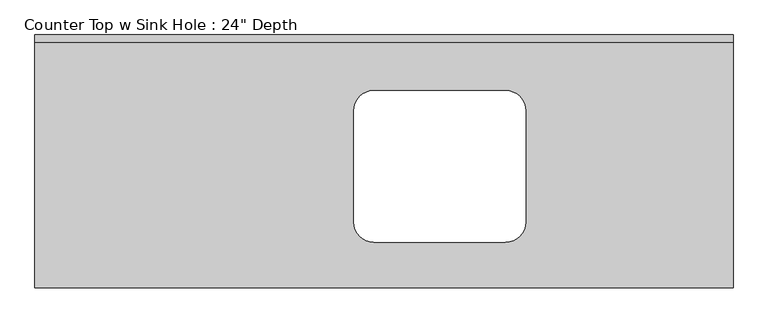
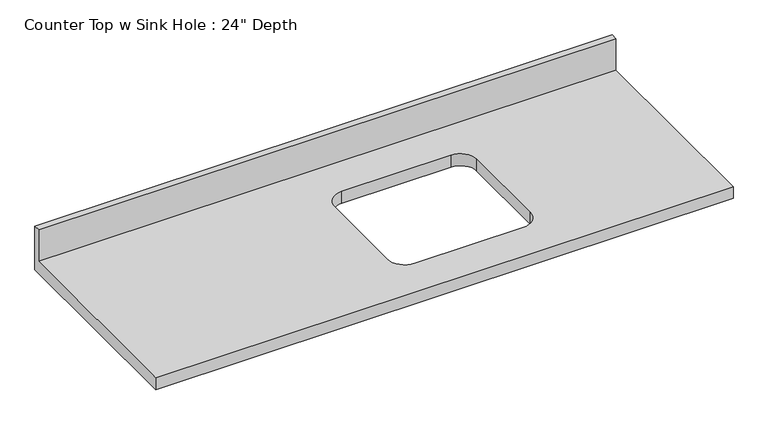
"""IFC4 building model written with IfcOpenShell, lengths in millimetres: furniture geometry."""

from ifc_helpers import new_model, si_unit, frame, origin, place, context, project, spatial, polyline, circle_curve, source, transform, mapped, element, save
from ifc_brep_helpers import plane_surface, revolved_surface, advanced_brep


def furniture_f14924cf(model_context):
    return source(origin(), model_context, "Body", "AdvancedBrep", [
        advanced_brep(
        [(-1200.4622951, -635.0, 914.4), (552.1377049, -635.0, 914.4), (552.1377049, -19.05, 914.4), (-1200.4622951, -19.05, 914.4), (-349.5622951, -139.7, 914.4), (-19.3622951, -139.7, 914.4), (31.4377049, -190.5, 914.4), (31.4377049, -469.9, 914.4), (-19.3622951, -520.7, 914.4), (-349.5622951, -520.7, 914.4), (-400.3622951, -469.9, 914.4), (-400.3622951, -190.5, 914.4), (552.1377049, 0.0, 876.3), (552.1377049, -635.0, 876.3), (-1200.4622951, -635.0, 876.3), (-1200.4622951, 0.0, 876.3), (-19.3622951, -139.7, 876.3), (-349.5622951, -139.7, 876.3), (-400.3622951, -190.5, 876.3), (-400.3622951, -469.9, 876.3), (-349.5622951, -520.7, 876.3), (-19.3622951, -520.7, 876.3), (31.4377049, -469.9, 876.3), (31.4377049, -190.5, 876.3), (-1200.4622951, 0.0, 1016.0), (552.1377049, 0.0, 1016.0), (-1200.4622951, -19.05, 1016.0), (552.1377049, -19.05, 1016.0)],
        [
            (0, 1),
            (1, 2),
            (2, 3),
            (3, 0),
            (4, 5),
            (5, 6, circle_curve(frame((-19.3622951, -190.5, 914.4), z_axis=(0.0, 0.0, -1.0), x_axis=(1.0, 0.0, 0.0)), 50.8)),
            (6, 7),
            (7, 8, circle_curve(frame((-19.3622951, -469.9, 914.4), z_axis=(0.0, 0.0, -1.0), x_axis=(1.0, 0.0, 0.0)), 50.8)),
            (8, 9),
            (9, 10, circle_curve(frame((-349.5622951, -469.9, 914.4), z_axis=(0.0, 0.0, -1.0), x_axis=(1.0, 0.0, 0.0)), 50.8)),
            (10, 11),
            (11, 4, circle_curve(frame((-349.5622951, -190.5, 914.4), z_axis=(0.0, 0.0, -1.0), x_axis=(1.0, 0.0, 0.0)), 50.8)),
            (12, 13),
            (13, 14),
            (14, 15),
            (15, 12),
            (16, 17),
            (17, 18, circle_curve(frame((-349.5622951, -190.5, 876.3), z_axis=(0.0, 0.0, 1.0), x_axis=(1.0, 0.0, 0.0)), 50.8)),
            (18, 19),
            (19, 20, circle_curve(frame((-349.5622951, -469.9, 876.3), z_axis=(0.0, 0.0, 1.0), x_axis=(1.0, 0.0, 0.0)), 50.8)),
            (20, 21),
            (21, 22, circle_curve(frame((-19.3622951, -469.9, 876.3), z_axis=(0.0, 0.0, 1.0), x_axis=(1.0, 0.0, 0.0)), 50.8)),
            (22, 23),
            (23, 16, circle_curve(frame((-19.3622951, -190.5, 876.3), z_axis=(0.0, 0.0, 1.0), x_axis=(1.0, 0.0, 0.0)), 50.8)),
            (15, 24),
            (24, 25),
            (25, 12),
            (14, 0),
            (3, 26),
            (26, 24),
            (13, 1),
            (25, 27),
            (27, 2),
            (4, 17),
            (16, 5),
            (11, 18),
            (10, 19),
            (9, 20),
            (8, 21),
            (7, 22),
            (6, 23),
            (26, 27),
        ],
        [
            plane_surface(frame((-1200.4622951, 0.0, 914.4), z_axis=(0.0, 0.0, 1.0), x_axis=(-1.0, 0.0, 0.0))),
            plane_surface(frame((-1200.4622951, 0.0, 876.3), z_axis=(0.0, 0.0, -1.0), x_axis=(1.0, 0.0, 0.0))),
            plane_surface(frame((552.1377049, 0.0, 914.4), z_axis=(0.0, 1.0, 0.0), x_axis=(0.0, 0.0, -1.0))),
            plane_surface(frame((-1200.4622951, 0.0, 914.4), z_axis=(-1.0, 0.0, 0.0), x_axis=(0.0, 0.0, -1.0))),
            plane_surface(frame((-1200.4622951, -635.0, 914.4), z_axis=(0.0, -1.0, 0.0), x_axis=(0.0, 0.0, -1.0))),
            plane_surface(frame((552.1377049, -635.0, 914.4), z_axis=(1.0, 0.0, 0.0), x_axis=(0.0, 0.0, -1.0))),
            plane_surface(frame((-19.3622951, -139.7, 914.4), z_axis=(0.0, -1.0, 0.0), x_axis=(0.0, 0.0, -1.0))),
            revolved_surface(polyline([(-298.76229509999996, -190.5, 914.4), (-298.76229509999996, -190.5, 876.3)]), (-349.5622951, -190.5, 876.3), (0.0, 0.0, 1.0)),
            plane_surface(frame((-400.3622951, -190.5, 914.4), z_axis=(1.0, 0.0, 0.0), x_axis=(0.0, 0.0, -1.0))),
            revolved_surface(polyline([(-298.76229509999996, -469.9, 914.4), (-298.76229509999996, -469.9, 876.3)]), (-349.5622951, -469.9, 876.3), (0.0, 0.0, 1.0)),
            plane_surface(frame((-349.5622951, -520.7, 914.4), z_axis=(0.0, 1.0, 0.0), x_axis=(0.0, 0.0, -1.0))),
            revolved_surface(polyline([(31.437704899999996, -469.9, 914.4), (31.437704899999996, -469.9, 876.3)]), (-19.3622951, -469.9, 876.3), (0.0, 0.0, 1.0)),
            plane_surface(frame((31.4377049, -469.9, 914.4), z_axis=(-1.0, 0.0, 0.0), x_axis=(0.0, 0.0, -1.0))),
            revolved_surface(polyline([(31.437704899999996, -190.5, 914.4), (31.437704899999996, -190.5, 876.3)]), (-19.3622951, -190.5, 876.3), (0.0, 0.0, 1.0)),
            plane_surface(frame((-1200.4622951, 0.0, 1016.0), z_axis=(0.0, 0.0, 1.0), x_axis=(0.0, -1.0, 0.0))),
            plane_surface(frame((-1200.4622951, -19.05, 1016.0), z_axis=(0.0, -1.0, 0.0), x_axis=(0.0, 0.0, -1.0))),
        ],
        [
            (0, [[1, 2, 3, 4], [5, 6, 7, 8, 9, 10, 11, 12]]),
            (1, [[13, 14, 15, 16], [17, 18, 19, 20, 21, 22, 23, 24]]),
            (2, [[-16, 25, 26, 27]]),
            (3, [[-15, 28, -4, 29, 30, -25]]),
            (4, [[-1, -28, -14, 31]]),
            (5, [[-13, -27, 32, 33, -2, -31]]),
            (6, [[34, -17, 35, -5]]),
            (7, [[-34, -12, 36, -18]]),
            (8, [[-36, -11, 37, -19]]),
            (9, [[-37, -10, 38, -20]]),
            (10, [[-38, -9, 39, -21]]),
            (11, [[-39, -8, 40, -22]]),
            (12, [[-40, -7, 41, -23]]),
            (13, [[-35, -24, -41, -6]]),
            (14, [[-30, 42, -32, -26]]),
            (15, [[-42, -29, -3, -33]]),
        ],
    ),
    ])


if __name__ == "__main__":
    model = new_model("IFC4")
    model_context = context("Model", 3, world=origin())
    ifc_project = project(units=[si_unit("LENGTHUNIT", "METRE", prefix="MILLI")], contexts=[model_context])
    site = spatial("IfcSite", under=ifc_project)
    building = spatial("IfcBuilding", under=site)
    placement = place(None, origin())
    furniture_shape = furniture_f14924cf(model_context)
    element("IfcFurniture", 1, ObjectType="Counter Top w Sink Hole : 24\" Depth", at=placement, inside=building, context=model_context, shape_type="MappedRepresentation", body=[
        mapped(furniture_shape, transform((0.0, 0.0, 0.0), x_axis=(1.0, 0.0, 0.0), y_axis=(0.0, 1.0, 0.0), z_axis=(0.0, 0.0, 1.0))),
    ])
    save(model, "model.ifc")

# Revit data of these elements
# Type "Counter Top w Sink Hole : 24\" Depth"
#   Assembly Code = "C1030400"
#   Counter Thickness = 0' - 1 1/2"
#   Depth = 2' - 1"
#   Height = 3' - 0"
#   Length [instance default] = 8' - 0"
#   Sink Location [instance default] = 2' - 0"
#   Sink Location To Wall [instance default] = 0' - 6"
#   Sink Opening Depth [instance default] = 1' - 3"
#   Sink Opening Width [instance default] = 2' - 3"
#   Counter Top Material = none
#   Default Elevation = 0
# Element 1 (IfcFurniture, "Counter Top w Sink Hole : 24\" Depth")
#   Length = 5' - 9"
#   Sink Location = 3' - 4"
#   Sink Opening Depth = 1' - 2"
#   Sink Opening Width = 1' - 4"
#   Materials on its faces: "Counter Top"
# Materials
#   "Counter Top": class "Wood", colour RGB 226 177 128, transparency 0
